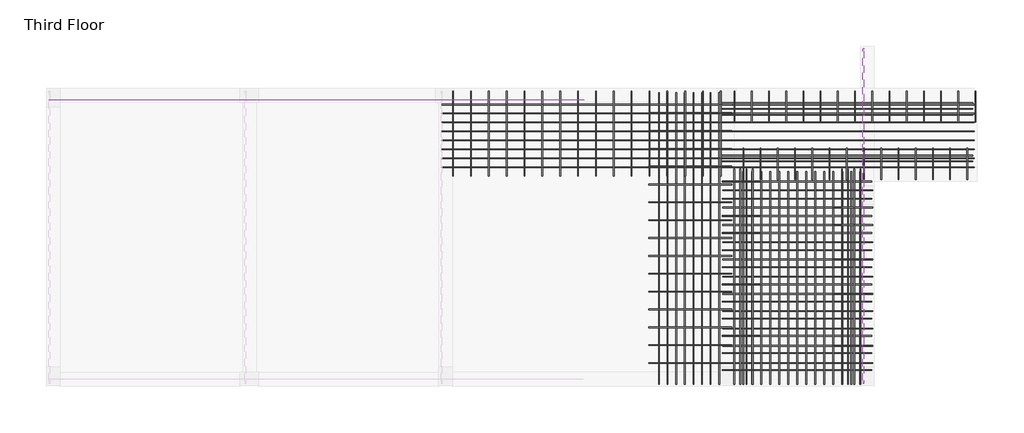
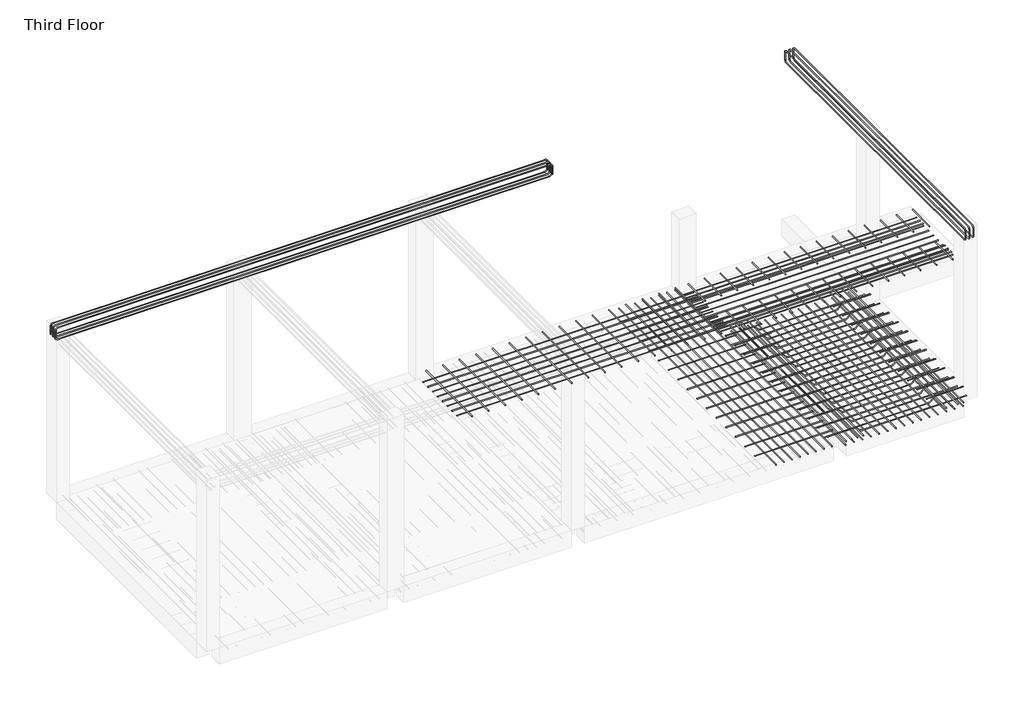
# One storey, part 4 of 4: 20 reinforcing bars.
"""IFC4 building model written with IfcOpenShell, lengths in millimetres."""

from ifc_helpers import new_model, si_unit, point, frame, origin, place, context, project, spatial, polyline, circle_curve, trimmed, segment, composite_curve, source, transform, mapped, element, save
from ifc_brep_helpers import swept_disk

model = new_model("IFC4")

# Units and contexts
model_context = context("Model", 3, world=origin())
ifc_project = project(units=[si_unit("LENGTHUNIT", "METRE", prefix="MILLI")], contexts=[model_context])

# Site, building, storey
site = spatial("IfcSite", under=ifc_project)
building = spatial("IfcBuilding", under=site)
storey = spatial("IfcBuildingStorey", under=building, Name="Third Floor", Elevation=9601.2)

# Reinforcing bars
placement = place(None, origin())
reinforcing_bar_shape = source(origin(), model_context, "Body", "SolidModel", [
    swept_disk(composite_curve([segment(polyline([(3999.1887526, 5724.7334631, 12564.4994949), (3999.1887526, 5724.7334631, 12712.4994949)]), True, "CONTINUOUS"), segment(trimmed(circle_curve(frame((3999.1887526, 5678.7334631, 12712.4994949), z_axis=(1.0, 0.0, 0.0), x_axis=(0.0, 46.0, 0.0)), 46.0), [point((3999.1887526, 5724.7334631, 12712.4994949))], [point((3999.1887526, 5678.7334631, 12758.4994949))], True, "CARTESIAN"), True, "CONTINUOUS"), segment(polyline([(3999.1887526, 5678.7334631, 12758.4994949), (3999.1887526, 278.4334631, 12758.4994949)]), True, "CONTINUOUS"), segment(trimmed(circle_curve(frame((3999.1887526, 278.4334631, 12712.4994949), z_axis=(1.0, 0.0, 0.0), x_axis=(0.0, 0.0, 46.0)), 46.0), [point((3999.1887526, 278.4334631, 12758.4994949))], [point((3999.1887526, 232.4334631, 12712.4994949))], True, "CARTESIAN"), True, "CONTINUOUS"), segment(polyline([(3999.1887526, 232.4334631, 12712.4994949), (3999.1887526, 232.4334631, 12564.4994949)]), True, "CONTINUOUS")], self_intersect=False), 6.0),
])
element("IfcReinforcingBar", 1, at=placement, inside=storey, context=model_context, shape_type="MappedRepresentation", body=[
    mapped(reinforcing_bar_shape, transform((0.0, 0.0, 0.0), x_axis=(1.0, 0.0, 0.0), y_axis=(0.0, 1.0, 0.0), z_axis=(0.0, 0.0, 1.0))),
    mapped(reinforcing_bar_shape, transform((71.1994949, 0.0, 0.0), x_axis=(1.0, 0.0, 0.0), y_axis=(0.0, 1.0, 0.0), z_axis=(0.0, 0.0, 1.0))),
    mapped(reinforcing_bar_shape, transform((142.3989899, 0.0, 0.0), x_axis=(1.0, 0.0, 0.0), y_axis=(0.0, 1.0, 0.0), z_axis=(0.0, 0.0, 1.0))),
])
reinforcing_bar_2_shape = source(origin(), model_context, "Body", "SolidModel", [
    swept_disk(composite_curve([segment(polyline([(3999.1887526, 5724.7334631, 12733.9005051), (3999.1887526, 5724.7334631, 12585.9005051)]), True, "CONTINUOUS"), segment(trimmed(circle_curve(frame((3999.1887526, 5678.7334631, 12585.9005051), z_axis=(-1.0, 0.0, 0.0), x_axis=(0.0, 46.0, 0.0)), 46.0), [point((3999.1887526, 5724.7334631, 12585.9005051))], [point((3999.1887526, 5678.7334631, 12539.9005051))], True, "CARTESIAN"), True, "CONTINUOUS"), segment(polyline([(3999.1887526, 5678.7334631, 12539.9005051), (3999.1887526, 278.4334631, 12539.9005051)]), True, "CONTINUOUS"), segment(trimmed(circle_curve(frame((3999.1887526, 278.4334631, 12585.9005051), z_axis=(-1.0, 0.0, 0.0), x_axis=(0.0, 0.0, -46.0)), 46.0), [point((3999.1887526, 278.4334631, 12539.9005051))], [point((3999.1887526, 232.4334631, 12585.9005051))], True, "CARTESIAN"), True, "CONTINUOUS"), segment(polyline([(3999.1887526, 232.4334631, 12585.9005051), (3999.1887526, 232.4334631, 12733.9005051)]), True, "CONTINUOUS")], self_intersect=False), 6.0),
])
element("IfcReinforcingBar", 2, at=placement, inside=storey, context=model_context, shape_type="MappedRepresentation", body=[
    mapped(reinforcing_bar_2_shape, transform((0.0, 0.0, 0.0), x_axis=(1.0, 0.0, 0.0), y_axis=(0.0, 1.0, 0.0), z_axis=(0.0, 0.0, 1.0))),
    mapped(reinforcing_bar_2_shape, transform((71.1994949, 0.0, 0.0), x_axis=(1.0, 0.0, 0.0), y_axis=(0.0, 1.0, 0.0), z_axis=(0.0, 0.0, 1.0))),
    mapped(reinforcing_bar_2_shape, transform((142.3989899, 0.0, 0.0), x_axis=(1.0, 0.0, 0.0), y_axis=(0.0, 1.0, 0.0), z_axis=(0.0, 0.0, 1.0))),
])
reinforcing_bar_3_shape = source(origin(), model_context, "Body", "SolidModel", [
    swept_disk(composite_curve([segment(polyline([(-586.8295875, 5020.132958, 12564.4994949), (-586.8295875, 5020.132958, 12712.4994949)]), True, "CONTINUOUS"), segment(trimmed(circle_curve(frame((-632.8295875, 5020.132958, 12712.4994949), z_axis=(0.0, -1.0, 0.0), x_axis=(46.0, 0.0, 0.0)), 46.0), [point((-586.8295875, 5020.132958, 12712.4994949))], [point((-632.8295875, 5020.132958, 12758.4994949))], True, "CARTESIAN"), True, "CONTINUOUS"), segment(polyline([(-632.8295875, 5020.132958, 12758.4994949), (-9286.9117524, 5020.132958, 12758.4994949)]), True, "CONTINUOUS"), segment(trimmed(circle_curve(frame((-9286.9117524, 5020.132958, 12712.4994949), z_axis=(0.0, -1.0, 0.0), x_axis=(0.0, 0.0, 46.0)), 46.0), [point((-9286.9117524, 5020.132958, 12758.4994949))], [point((-9332.9117524, 5020.132958, 12712.4994949))], True, "CARTESIAN"), True, "CONTINUOUS"), segment(polyline([(-9332.9117524, 5020.132958, 12712.4994949), (-9332.9117524, 5020.132958, 12564.4994949)]), True, "CONTINUOUS")], self_intersect=False), 6.0),
])
element("IfcReinforcingBar", 3, at=placement, inside=storey, context=model_context, shape_type="MappedRepresentation", body=[
    mapped(reinforcing_bar_3_shape, transform((0.0, 0.0, 0.0), x_axis=(1.0, 0.0, 0.0), y_axis=(0.0, 1.0, 0.0), z_axis=(0.0, 0.0, 1.0))),
    mapped(reinforcing_bar_3_shape, transform((0.0, -71.1994949, 0.0), x_axis=(1.0, 0.0, 0.0), y_axis=(0.0, 1.0, 0.0), z_axis=(0.0, 0.0, 1.0))),
    mapped(reinforcing_bar_3_shape, transform((0.0, -142.3989899, 0.0), x_axis=(1.0, 0.0, 0.0), y_axis=(0.0, 1.0, 0.0), z_axis=(0.0, 0.0, 1.0))),
])
reinforcing_bar_4_shape = source(origin(), model_context, "Body", "SolidModel", [
    swept_disk(composite_curve([segment(polyline([(-596.1117524, 5020.132958, 12733.9005051), (-596.1117524, 5020.132958, 12585.9005051)]), True, "CONTINUOUS"), segment(trimmed(circle_curve(frame((-642.1117524, 5020.132958, 12585.9005051), z_axis=(0.0, 1.0, 0.0), x_axis=(46.0, 0.0, 0.0)), 46.0), [point((-596.1117524, 5020.132958, 12585.9005051))], [point((-642.1117524, 5020.132958, 12539.9005051))], True, "CARTESIAN"), True, "CONTINUOUS"), segment(polyline([(-642.1117524, 5020.132958, 12539.9005051), (-9277.4938356, 5020.132958, 12539.9005051)]), True, "CONTINUOUS"), segment(trimmed(circle_curve(frame((-9277.4938356, 5020.132958, 12585.9005051), z_axis=(0.0, 1.0, 0.0), x_axis=(0.0, 0.0, -46.0)), 46.0), [point((-9277.4938356, 5020.132958, 12539.9005051))], [point((-9323.4938356, 5020.132958, 12585.9005051))], True, "CARTESIAN"), True, "CONTINUOUS"), segment(polyline([(-9323.4938356, 5020.132958, 12585.9005051), (-9323.4938356, 5020.132958, 12733.9005051)]), True, "CONTINUOUS")], self_intersect=False), 6.0),
])
element("IfcReinforcingBar", 4, at=placement, inside=storey, context=model_context, shape_type="MappedRepresentation", body=[
    mapped(reinforcing_bar_4_shape, transform((0.0, 0.0, 0.0), x_axis=(1.0, 0.0, 0.0), y_axis=(0.0, 1.0, 0.0), z_axis=(0.0, 0.0, 1.0))),
    mapped(reinforcing_bar_4_shape, transform((0.0, -71.1994949, 0.0), x_axis=(1.0, 0.0, 0.0), y_axis=(0.0, 1.0, 0.0), z_axis=(0.0, 0.0, 1.0))),
    mapped(reinforcing_bar_4_shape, transform((0.0, -142.3989899, 0.0), x_axis=(1.0, 0.0, 0.0), y_axis=(0.0, 1.0, 0.0), z_axis=(0.0, 0.0, 1.0))),
])
reinforcing_bar_5_shape = source(origin(), model_context, "Body", "SolidModel", [
    swept_disk(composite_curve([segment(polyline([(1688.7874305, 3539.2334631, 9570.2), (2168.5956769, 3539.2334631, 9570.2)]), True, "CONTINUOUS"), segment(trimmed(circle_curve(frame((2168.5956769, 3539.2334631, 9524.2), z_axis=(0.0, 1.0, 0.0), x_axis=(0.0, 0.0, 46.0)), 46.0), [point((2168.5956769, 3539.2334631, 9570.2))], [point((2201.1225888, 3539.2334631, 9556.7269119))], True, "CARTESIAN"), True, "CONTINUOUS"), segment(polyline([(2201.1225888, 3539.2334631, 9556.7269119), (2264.5764127, 3539.2334631, 9493.2730881)]), True, "CONTINUOUS"), segment(trimmed(circle_curve(frame((2297.1033246, 3539.2334631, 9525.8), z_axis=(0.0, -1.0, 0.0), x_axis=(-32.52691189999996, 0.0, -32.526911899998595)), 46.0), [point((2264.5764127, 3539.2334631, 9493.2730881))], [point((2297.1033246, 3539.2334631, 9479.8))], True, "CARTESIAN"), True, "CONTINUOUS"), segment(polyline([(2297.1033246, 3539.2334631, 9479.8), (4139.8402551, 3539.2334631, 9479.8)]), True, "CONTINUOUS")], self_intersect=False), 6.0),
])
element("IfcReinforcingBar", 5, at=placement, inside=storey, context=model_context, shape_type="MappedRepresentation", body=[
    mapped(reinforcing_bar_5_shape, transform((0.0, 0.0, 0.0), x_axis=(1.0, 0.0, 0.0), y_axis=(0.0, 1.0, 0.0), z_axis=(0.0, 0.0, 1.0))),
    mapped(reinforcing_bar_5_shape, transform((0.0, -281.0909091, 0.0), x_axis=(1.0, 0.0, 0.0), y_axis=(0.0, 1.0, 0.0), z_axis=(0.0, 0.0, 1.0))),
    mapped(reinforcing_bar_5_shape, transform((0.0, -562.1818182, 0.0), x_axis=(1.0, 0.0, 0.0), y_axis=(0.0, 1.0, 0.0), z_axis=(0.0, 0.0, 1.0))),
    mapped(reinforcing_bar_5_shape, transform((0.0, -843.2727273, 0.0), x_axis=(1.0, 0.0, 0.0), y_axis=(0.0, 1.0, 0.0), z_axis=(0.0, 0.0, 1.0))),
    mapped(reinforcing_bar_5_shape, transform((0.0, -1124.3636364, 0.0), x_axis=(1.0, 0.0, 0.0), y_axis=(0.0, 1.0, 0.0), z_axis=(0.0, 0.0, 1.0))),
    mapped(reinforcing_bar_5_shape, transform((0.0, -1405.4545455, 0.0), x_axis=(1.0, 0.0, 0.0), y_axis=(0.0, 1.0, 0.0), z_axis=(0.0, 0.0, 1.0))),
    mapped(reinforcing_bar_5_shape, transform((0.0, -1686.5454545, 0.0), x_axis=(1.0, 0.0, 0.0), y_axis=(0.0, 1.0, 0.0), z_axis=(0.0, 0.0, 1.0))),
    mapped(reinforcing_bar_5_shape, transform((0.0, -1967.6363636, 0.0), x_axis=(1.0, 0.0, 0.0), y_axis=(0.0, 1.0, 0.0), z_axis=(0.0, 0.0, 1.0))),
    mapped(reinforcing_bar_5_shape, transform((0.0, -2248.7272727, 0.0), x_axis=(1.0, 0.0, 0.0), y_axis=(0.0, 1.0, 0.0), z_axis=(0.0, 0.0, 1.0))),
    mapped(reinforcing_bar_5_shape, transform((0.0, -2529.8181818, 0.0), x_axis=(1.0, 0.0, 0.0), y_axis=(0.0, 1.0, 0.0), z_axis=(0.0, 0.0, 1.0))),
    mapped(reinforcing_bar_5_shape, transform((0.0, -2810.9090909, 0.0), x_axis=(1.0, 0.0, 0.0), y_axis=(0.0, 1.0, 0.0), z_axis=(0.0, 0.0, 1.0))),
    mapped(reinforcing_bar_5_shape, transform((0.0, -3092.0, 0.0), x_axis=(1.0, 0.0, 0.0), y_axis=(0.0, 1.0, 0.0), z_axis=(0.0, 0.0, 1.0))),
])
reinforcing_bar_6_shape = source(origin(), model_context, "Body", "SolidModel", [
    swept_disk(composite_curve([segment(polyline([(4153.2890646, 564.2307141, 9570.2), (3672.2951557, 564.2307141, 9570.2)]), True, "CONTINUOUS"), segment(trimmed(circle_curve(frame((3672.2951557, 564.2307141, 9524.2), z_axis=(0.0, -1.0, 0.0), x_axis=(0.0, 0.0, 46.0)), 46.0), [point((3672.2951557, 564.2307141, 9570.2))], [point((3639.7682438, 564.2307141, 9556.7269119))], True, "CARTESIAN"), True, "CONTINUOUS"), segment(polyline([(3639.7682438, 564.2307141, 9556.7269119), (3576.3144199, 564.2307141, 9493.2730881)]), True, "CONTINUOUS"), segment(trimmed(circle_curve(frame((3543.787508, 564.2307141, 9525.8), z_axis=(0.0, 1.0000000000000002, 0.0), x_axis=(32.52691189999996, 0.0, -32.526911899998595)), 46.0), [point((3576.3144199, 564.2307141, 9493.2730881))], [point((3543.787508, 564.2307141, 9479.8))], True, "CARTESIAN"), True, "CONTINUOUS"), segment(polyline([(3543.787508, 564.2307141, 9479.8), (1702.23624, 564.2307141, 9479.8)]), True, "CONTINUOUS")], self_intersect=False), 6.0),
])
element("IfcReinforcingBar", 6, at=placement, inside=storey, context=model_context, shape_type="MappedRepresentation", body=[
    mapped(reinforcing_bar_6_shape, transform((0.0, 0.0, 0.0), x_axis=(1.0, 0.0, 0.0), y_axis=(0.0, 1.0, 0.0), z_axis=(0.0, 0.0, 1.0))),
    mapped(reinforcing_bar_6_shape, transform((0.0, 283.1945647, 0.0), x_axis=(1.0, 0.0, 0.0), y_axis=(0.0, 1.0, 0.0), z_axis=(0.0, 0.0, 1.0))),
    mapped(reinforcing_bar_6_shape, transform((0.0, 566.3891295, 0.0), x_axis=(1.0, 0.0, 0.0), y_axis=(0.0, 1.0, 0.0), z_axis=(0.0, 0.0, 1.0))),
    mapped(reinforcing_bar_6_shape, transform((0.0, 849.5836942, 0.0), x_axis=(1.0, 0.0, 0.0), y_axis=(0.0, 1.0, 0.0), z_axis=(0.0, 0.0, 1.0))),
    mapped(reinforcing_bar_6_shape, transform((0.0, 1132.778259, 0.0), x_axis=(1.0, 0.0, 0.0), y_axis=(0.0, 1.0, 0.0), z_axis=(0.0, 0.0, 1.0))),
    mapped(reinforcing_bar_6_shape, transform((0.0, 1415.9728237, 0.0), x_axis=(1.0, 0.0, 0.0), y_axis=(0.0, 1.0, 0.0), z_axis=(0.0, 0.0, 1.0))),
    mapped(reinforcing_bar_6_shape, transform((0.0, 1699.1673885, 0.0), x_axis=(1.0, 0.0, 0.0), y_axis=(0.0, 1.0, 0.0), z_axis=(0.0, 0.0, 1.0))),
    mapped(reinforcing_bar_6_shape, transform((0.0, 1982.3619532, 0.0), x_axis=(1.0, 0.0, 0.0), y_axis=(0.0, 1.0, 0.0), z_axis=(0.0, 0.0, 1.0))),
    mapped(reinforcing_bar_6_shape, transform((0.0, 2265.556518, 0.0), x_axis=(1.0, 0.0, 0.0), y_axis=(0.0, 1.0, 0.0), z_axis=(0.0, 0.0, 1.0))),
    mapped(reinforcing_bar_6_shape, transform((0.0, 2548.7510827, 0.0), x_axis=(1.0, 0.0, 0.0), y_axis=(0.0, 1.0, 0.0), z_axis=(0.0, 0.0, 1.0))),
    mapped(reinforcing_bar_6_shape, transform((0.0, 2831.9456475, 0.0), x_axis=(1.0, 0.0, 0.0), y_axis=(0.0, 1.0, 0.0), z_axis=(0.0, 0.0, 1.0))),
])
reinforcing_bar_7_shape = source(origin(), model_context, "Body", "SolidModel", [
    swept_disk(composite_curve([segment(polyline([(3650.7560505, 3742.8334631, 9559.9006995), (3650.7560505, 211.4334631, 9559.9006995)]), True, "CONTINUOUS")], self_intersect=False), 6.0),
])
element("IfcReinforcingBar", 7, at=placement, inside=storey, context=model_context, shape_type="MappedRepresentation", body=[
    mapped(reinforcing_bar_7_shape, transform((0.0, 0.0, 0.0), x_axis=(1.0, 0.0, 0.0), y_axis=(0.0, 1.0, 0.0), z_axis=(0.0, 0.0, 1.0))),
    mapped(reinforcing_bar_7_shape, transform((101.777399, 0.0, 0.0), x_axis=(1.0, 0.0, 0.0), y_axis=(0.0, 1.0, 0.0), z_axis=(0.0, 0.0, 1.0))),
    mapped(reinforcing_bar_7_shape, transform((203.554798, 0.0, 0.0), x_axis=(1.0, 0.0, 0.0), y_axis=(0.0, 1.0, 0.0), z_axis=(0.0, 0.0, 1.0))),
    mapped(reinforcing_bar_7_shape, transform((305.3321971, 0.0, 0.0), x_axis=(1.0, 0.0, 0.0), y_axis=(0.0, 1.0, 0.0), z_axis=(0.0, 0.0, 1.0))),
])
reinforcing_bar_8_shape = source(origin(), model_context, "Body", "SolidModel", [
    swept_disk(composite_curve([segment(polyline([(1697.8477074, 3539.2334631, 9572.2), (2325.3671503, 3539.2334631, 9572.2)]), True, "CONTINUOUS")], self_intersect=False), 4.0),
])
element("IfcReinforcingBar", 8, at=placement, inside=storey, context=model_context, shape_type="MappedRepresentation", body=[
    mapped(reinforcing_bar_8_shape, transform((0.0, 0.0, 0.0), x_axis=(1.0, 0.0, 0.0), y_axis=(0.0, 1.0, 0.0), z_axis=(0.0, 0.0, 1.0))),
    mapped(reinforcing_bar_8_shape, transform((0.0, -281.0909091, 0.0), x_axis=(1.0, 0.0, 0.0), y_axis=(0.0, 1.0, 0.0), z_axis=(0.0, 0.0, 1.0))),
    mapped(reinforcing_bar_8_shape, transform((0.0, -562.1818182, 0.0), x_axis=(1.0, 0.0, 0.0), y_axis=(0.0, 1.0, 0.0), z_axis=(0.0, 0.0, 1.0))),
    mapped(reinforcing_bar_8_shape, transform((0.0, -843.2727273, 0.0), x_axis=(1.0, 0.0, 0.0), y_axis=(0.0, 1.0, 0.0), z_axis=(0.0, 0.0, 1.0))),
    mapped(reinforcing_bar_8_shape, transform((0.0, -1124.3636364, 0.0), x_axis=(1.0, 0.0, 0.0), y_axis=(0.0, 1.0, 0.0), z_axis=(0.0, 0.0, 1.0))),
    mapped(reinforcing_bar_8_shape, transform((0.0, -1405.4545455, 0.0), x_axis=(1.0, 0.0, 0.0), y_axis=(0.0, 1.0, 0.0), z_axis=(0.0, 0.0, 1.0))),
    mapped(reinforcing_bar_8_shape, transform((0.0, -1686.5454545, 0.0), x_axis=(1.0, 0.0, 0.0), y_axis=(0.0, 1.0, 0.0), z_axis=(0.0, 0.0, 1.0))),
    mapped(reinforcing_bar_8_shape, transform((0.0, -1967.6363636, 0.0), x_axis=(1.0, 0.0, 0.0), y_axis=(0.0, 1.0, 0.0), z_axis=(0.0, 0.0, 1.0))),
    mapped(reinforcing_bar_8_shape, transform((0.0, -2248.7272727, 0.0), x_axis=(1.0, 0.0, 0.0), y_axis=(0.0, 1.0, 0.0), z_axis=(0.0, 0.0, 1.0))),
    mapped(reinforcing_bar_8_shape, transform((0.0, -2529.8181818, 0.0), x_axis=(1.0, 0.0, 0.0), y_axis=(0.0, 1.0, 0.0), z_axis=(0.0, 0.0, 1.0))),
    mapped(reinforcing_bar_8_shape, transform((0.0, -2810.9090909, 0.0), x_axis=(1.0, 0.0, 0.0), y_axis=(0.0, 1.0, 0.0), z_axis=(0.0, 0.0, 1.0))),
    mapped(reinforcing_bar_8_shape, transform((0.0, -3092.0, 0.0), x_axis=(1.0, 0.0, 0.0), y_axis=(0.0, 1.0, 0.0), z_axis=(0.0, 0.0, 1.0))),
])
reinforcing_bar_9_shape = source(origin(), model_context, "Body", "SolidModel", [
    swept_disk(composite_curve([segment(polyline([(4130.5876361, 3396.1763616, 9572.2), (3500.3340616, 3396.1763616, 9572.2)]), True, "CONTINUOUS")], self_intersect=False), 4.0),
])
element("IfcReinforcingBar", 9, at=placement, inside=storey, context=model_context, shape_type="MappedRepresentation", body=[
    mapped(reinforcing_bar_9_shape, transform((0.0, 0.0, 0.0), x_axis=(1.0, 0.0, 0.0), y_axis=(0.0, 1.0, 0.0), z_axis=(0.0, 0.0, 1.0))),
    mapped(reinforcing_bar_9_shape, transform((0.0, -283.1945647, 0.0), x_axis=(1.0, 0.0, 0.0), y_axis=(0.0, 1.0, 0.0), z_axis=(0.0, 0.0, 1.0))),
    mapped(reinforcing_bar_9_shape, transform((0.0, -566.3891295, 0.0), x_axis=(1.0, 0.0, 0.0), y_axis=(0.0, 1.0, 0.0), z_axis=(0.0, 0.0, 1.0))),
    mapped(reinforcing_bar_9_shape, transform((0.0, -849.5836942, 0.0), x_axis=(1.0, 0.0, 0.0), y_axis=(0.0, 1.0, 0.0), z_axis=(0.0, 0.0, 1.0))),
    mapped(reinforcing_bar_9_shape, transform((0.0, -1132.778259, 0.0), x_axis=(1.0, 0.0, 0.0), y_axis=(0.0, 1.0, 0.0), z_axis=(0.0, 0.0, 1.0))),
    mapped(reinforcing_bar_9_shape, transform((0.0, -1415.9728237, 0.0), x_axis=(1.0, 0.0, 0.0), y_axis=(0.0, 1.0, 0.0), z_axis=(0.0, 0.0, 1.0))),
    mapped(reinforcing_bar_9_shape, transform((0.0, -1699.1673885, 0.0), x_axis=(1.0, 0.0, 0.0), y_axis=(0.0, 1.0, 0.0), z_axis=(0.0, 0.0, 1.0))),
    mapped(reinforcing_bar_9_shape, transform((0.0, -1982.3619532, 0.0), x_axis=(1.0, 0.0, 0.0), y_axis=(0.0, 1.0, 0.0), z_axis=(0.0, 0.0, 1.0))),
    mapped(reinforcing_bar_9_shape, transform((0.0, -2265.556518, 0.0), x_axis=(1.0, 0.0, 0.0), y_axis=(0.0, 1.0, 0.0), z_axis=(0.0, 0.0, 1.0))),
    mapped(reinforcing_bar_9_shape, transform((0.0, -2548.7510827, 0.0), x_axis=(1.0, 0.0, 0.0), y_axis=(0.0, 1.0, 0.0), z_axis=(0.0, 0.0, 1.0))),
    mapped(reinforcing_bar_9_shape, transform((0.0, -2831.9456475, 0.0), x_axis=(1.0, 0.0, 0.0), y_axis=(0.0, 1.0, 0.0), z_axis=(0.0, 0.0, 1.0))),
])
reinforcing_bar_10_shape = source(origin(), model_context, "Body", "SolidModel", [
    swept_disk(composite_curve([segment(polyline([(3952.0882476, 218.9117605, 9488.3387401), (3952.0882476, 3706.6679133, 9488.3387401)]), True, "CONTINUOUS")], self_intersect=False), 6.0),
])
element("IfcReinforcingBar", 10, at=placement, inside=storey, context=model_context, shape_type="MappedRepresentation", body=[
    mapped(reinforcing_bar_10_shape, transform((0.0, 0.0, 0.0), x_axis=(1.0, 0.0, 0.0), y_axis=(0.0, 1.0, 0.0), z_axis=(0.0, 0.0, 1.0))),
    mapped(reinforcing_bar_10_shape, transform((-147.5785714, 0.0, 0.0), x_axis=(1.0, 0.0, 0.0), y_axis=(0.0, 1.0, 0.0), z_axis=(0.0, 0.0, 1.0))),
    mapped(reinforcing_bar_10_shape, transform((-295.1571429, 0.0, 0.0), x_axis=(1.0, 0.0, 0.0), y_axis=(0.0, 1.0, 0.0), z_axis=(0.0, 0.0, 1.0))),
    mapped(reinforcing_bar_10_shape, transform((-442.7357143, 0.0, 0.0), x_axis=(1.0, 0.0, 0.0), y_axis=(0.0, 1.0, 0.0), z_axis=(0.0, 0.0, 1.0))),
    mapped(reinforcing_bar_10_shape, transform((-590.3142857, 0.0, 0.0), x_axis=(1.0, 0.0, 0.0), y_axis=(0.0, 1.0, 0.0), z_axis=(0.0, 0.0, 1.0))),
    mapped(reinforcing_bar_10_shape, transform((-737.8928571, 0.0, 0.0), x_axis=(1.0, 0.0, 0.0), y_axis=(0.0, 1.0, 0.0), z_axis=(0.0, 0.0, 1.0))),
    mapped(reinforcing_bar_10_shape, transform((-885.4714286, 0.0, 0.0), x_axis=(1.0, 0.0, 0.0), y_axis=(0.0, 1.0, 0.0), z_axis=(0.0, 0.0, 1.0))),
    mapped(reinforcing_bar_10_shape, transform((-1033.05, 0.0, 0.0), x_axis=(1.0, 0.0, 0.0), y_axis=(0.0, 1.0, 0.0), z_axis=(0.0, 0.0, 1.0))),
    mapped(reinforcing_bar_10_shape, transform((-1180.6285714, 0.0, 0.0), x_axis=(1.0, 0.0, 0.0), y_axis=(0.0, 1.0, 0.0), z_axis=(0.0, 0.0, 1.0))),
    mapped(reinforcing_bar_10_shape, transform((-1328.2071429, 0.0, 0.0), x_axis=(1.0, 0.0, 0.0), y_axis=(0.0, 1.0, 0.0), z_axis=(0.0, 0.0, 1.0))),
    mapped(reinforcing_bar_10_shape, transform((-1475.7857143, 0.0, 0.0), x_axis=(1.0, 0.0, 0.0), y_axis=(0.0, 1.0, 0.0), z_axis=(0.0, 0.0, 1.0))),
    mapped(reinforcing_bar_10_shape, transform((-1623.3642857, 0.0, 0.0), x_axis=(1.0, 0.0, 0.0), y_axis=(0.0, 1.0, 0.0), z_axis=(0.0, 0.0, 1.0))),
    mapped(reinforcing_bar_10_shape, transform((-1770.9428571, 0.0, 0.0), x_axis=(1.0, 0.0, 0.0), y_axis=(0.0, 1.0, 0.0), z_axis=(0.0, 0.0, 1.0))),
    mapped(reinforcing_bar_10_shape, transform((-1918.5214286, 0.0, 0.0), x_axis=(1.0, 0.0, 0.0), y_axis=(0.0, 1.0, 0.0), z_axis=(0.0, 0.0, 1.0))),
    mapped(reinforcing_bar_10_shape, transform((-2066.1, 0.0, 0.0), x_axis=(1.0, 0.0, 0.0), y_axis=(0.0, 1.0, 0.0), z_axis=(0.0, 0.0, 1.0))),
])
reinforcing_bar_11_shape = source(origin(), model_context, "Body", "SolidModel", [
    swept_disk(composite_curve([segment(polyline([(2190.1347821, 3742.8334631, 9559.9006995), (2190.1347821, 211.4334631, 9559.9006995)]), True, "CONTINUOUS")], self_intersect=False), 6.0),
])
element("IfcReinforcingBar", 11, at=placement, inside=storey, context=model_context, shape_type="MappedRepresentation", body=[
    mapped(reinforcing_bar_11_shape, transform((0.0, 0.0, 0.0), x_axis=(1.0, 0.0, 0.0), y_axis=(0.0, 1.0, 0.0), z_axis=(0.0, 0.0, 1.0))),
    mapped(reinforcing_bar_11_shape, transform((-101.3821782, 0.0, 0.0), x_axis=(1.0, 0.0, 0.0), y_axis=(0.0, 1.0, 0.0), z_axis=(0.0, 0.0, 1.0))),
    mapped(reinforcing_bar_11_shape, transform((-202.7643564, 0.0, 0.0), x_axis=(1.0, 0.0, 0.0), y_axis=(0.0, 1.0, 0.0), z_axis=(0.0, 0.0, 1.0))),
    mapped(reinforcing_bar_11_shape, transform((-304.1465345, 0.0, 0.0), x_axis=(1.0, 0.0, 0.0), y_axis=(0.0, 1.0, 0.0), z_axis=(0.0, 0.0, 1.0))),
])
reinforcing_bar_12_shape = source(origin(), model_context, "Body", "SolidModel", [
    swept_disk(composite_curve([segment(polyline([(654.4332967, 4999.0798317, 9555.2697281), (654.4332967, 211.4334631, 9555.2697281)]), True, "CONTINUOUS")], self_intersect=False), 6.0),
])
element("IfcReinforcingBar", 12, at=placement, inside=storey, context=model_context, shape_type="MappedRepresentation", body=[
    mapped(reinforcing_bar_12_shape, transform((0.0, 0.0, 0.0), x_axis=(1.0, 0.0, 0.0), y_axis=(0.0, 1.0, 0.0), z_axis=(0.0, 0.0, 1.0))),
    mapped(reinforcing_bar_12_shape, transform((140.8412233, 0.0, 0.0), x_axis=(1.0, 0.0, 0.0), y_axis=(0.0, 1.0, 0.0), z_axis=(0.0, 0.0, 1.0))),
    mapped(reinforcing_bar_12_shape, transform((281.6824466, 0.0, 0.0), x_axis=(1.0, 0.0, 0.0), y_axis=(0.0, 1.0, 0.0), z_axis=(0.0, 0.0, 1.0))),
    mapped(reinforcing_bar_12_shape, transform((422.5236699, 0.0, 0.0), x_axis=(1.0, 0.0, 0.0), y_axis=(0.0, 1.0, 0.0), z_axis=(0.0, 0.0, 1.0))),
    mapped(reinforcing_bar_12_shape, transform((563.3648932, 0.0, 0.0), x_axis=(1.0, 0.0, 0.0), y_axis=(0.0, 1.0, 0.0), z_axis=(0.0, 0.0, 1.0))),
    mapped(reinforcing_bar_12_shape, transform((704.2061164, 0.0, 0.0), x_axis=(1.0, 0.0, 0.0), y_axis=(0.0, 1.0, 0.0), z_axis=(0.0, 0.0, 1.0))),
    mapped(reinforcing_bar_12_shape, transform((845.0473397, 0.0, 0.0), x_axis=(1.0, 0.0, 0.0), y_axis=(0.0, 1.0, 0.0), z_axis=(0.0, 0.0, 1.0))),
    mapped(reinforcing_bar_12_shape, transform((985.888563, 0.0, 0.0), x_axis=(1.0, 0.0, 0.0), y_axis=(0.0, 1.0, 0.0), z_axis=(0.0, 0.0, 1.0))),
])
reinforcing_bar_13_shape = source(origin(), model_context, "Body", "SolidModel", [
    swept_disk(composite_curve([segment(polyline([(1844.9074635, 564.2307141, 9564.6017937), (483.2910842, 564.2307141, 9564.6017937)]), True, "CONTINUOUS")], self_intersect=False), 6.0),
])
element("IfcReinforcingBar", 13, at=placement, inside=storey, context=model_context, shape_type="MappedRepresentation", body=[
    mapped(reinforcing_bar_13_shape, transform((0.0, 0.0, 0.0), x_axis=(1.0, 0.0, 0.0), y_axis=(0.0, 1.0, 0.0), z_axis=(0.0, 0.0, 1.0))),
    mapped(reinforcing_bar_13_shape, transform((0.0, 292.7783831, 0.0), x_axis=(1.0, 0.0, 0.0), y_axis=(0.0, 1.0, 0.0), z_axis=(0.0, 0.0, 1.0))),
    mapped(reinforcing_bar_13_shape, transform((0.0, 585.5567661, 0.0), x_axis=(1.0, 0.0, 0.0), y_axis=(0.0, 1.0, 0.0), z_axis=(0.0, 0.0, 1.0))),
    mapped(reinforcing_bar_13_shape, transform((0.0, 878.3351492, 0.0), x_axis=(1.0, 0.0, 0.0), y_axis=(0.0, 1.0, 0.0), z_axis=(0.0, 0.0, 1.0))),
    mapped(reinforcing_bar_13_shape, transform((0.0, 1171.1135323, 0.0), x_axis=(1.0, 0.0, 0.0), y_axis=(0.0, 1.0, 0.0), z_axis=(0.0, 0.0, 1.0))),
    mapped(reinforcing_bar_13_shape, transform((0.0, 1463.8919154, 0.0), x_axis=(1.0, 0.0, 0.0), y_axis=(0.0, 1.0, 0.0), z_axis=(0.0, 0.0, 1.0))),
    mapped(reinforcing_bar_13_shape, transform((0.0, 1756.6702984, 0.0), x_axis=(1.0, 0.0, 0.0), y_axis=(0.0, 1.0, 0.0), z_axis=(0.0, 0.0, 1.0))),
    mapped(reinforcing_bar_13_shape, transform((0.0, 2049.4486815, 0.0), x_axis=(1.0, 0.0, 0.0), y_axis=(0.0, 1.0, 0.0), z_axis=(0.0, 0.0, 1.0))),
    mapped(reinforcing_bar_13_shape, transform((0.0, 2342.2270646, 0.0), x_axis=(1.0, 0.0, 0.0), y_axis=(0.0, 1.0, 0.0), z_axis=(0.0, 0.0, 1.0))),
    mapped(reinforcing_bar_13_shape, transform((0.0, 2635.0054477, 0.0), x_axis=(1.0, 0.0, 0.0), y_axis=(0.0, 1.0, 0.0), z_axis=(0.0, 0.0, 1.0))),
    mapped(reinforcing_bar_13_shape, transform((0.0, 2927.7838307, 0.0), x_axis=(1.0, 0.0, 0.0), y_axis=(0.0, 1.0, 0.0), z_axis=(0.0, 0.0, 1.0))),
    mapped(reinforcing_bar_13_shape, transform((0.0, 3220.5622138, 0.0), x_axis=(1.0, 0.0, 0.0), y_axis=(0.0, 1.0, 0.0), z_axis=(0.0, 0.0, 1.0))),
    mapped(reinforcing_bar_13_shape, transform((0.0, 3513.3405969, 0.0), x_axis=(1.0, 0.0, 0.0), y_axis=(0.0, 1.0, 0.0), z_axis=(0.0, 0.0, 1.0))),
    mapped(reinforcing_bar_13_shape, transform((0.0, 3806.11898, 0.0), x_axis=(1.0, 0.0, 0.0), y_axis=(0.0, 1.0, 0.0), z_axis=(0.0, 0.0, 1.0))),
    mapped(reinforcing_bar_13_shape, transform((0.0, 4098.897363, 0.0), x_axis=(1.0, 0.0, 0.0), y_axis=(0.0, 1.0, 0.0), z_axis=(0.0, 0.0, 1.0))),
])
reinforcing_bar_14_shape = source(origin(), model_context, "Body", "SolidModel", [
    swept_disk(composite_curve([segment(polyline([(1854.5084921, 3775.4003908, 9554.9006995), (-2903.4807845, 3775.4003908, 9554.9006995)]), True, "CONTINUOUS")], self_intersect=False), 6.0),
])
element("IfcReinforcingBar", 14, at=placement, inside=storey, context=model_context, shape_type="MappedRepresentation", body=[
    mapped(reinforcing_bar_14_shape, transform((0.0, 0.0, 0.0), x_axis=(1.0, 0.0, 0.0), y_axis=(0.0, 1.0, 0.0), z_axis=(0.0, 0.0, 1.0))),
    mapped(reinforcing_bar_14_shape, transform((0.0, 146.8904389, 0.0), x_axis=(1.0, 0.0, 0.0), y_axis=(0.0, 1.0, 0.0), z_axis=(0.0, 0.0, 1.0))),
    mapped(reinforcing_bar_14_shape, transform((0.0, 293.7808778, 0.0), x_axis=(1.0, 0.0, 0.0), y_axis=(0.0, 1.0, 0.0), z_axis=(0.0, 0.0, 1.0))),
    mapped(reinforcing_bar_14_shape, transform((0.0, 440.6713167, 0.0), x_axis=(1.0, 0.0, 0.0), y_axis=(0.0, 1.0, 0.0), z_axis=(0.0, 0.0, 1.0))),
    mapped(reinforcing_bar_14_shape, transform((0.0, 587.5617556, 0.0), x_axis=(1.0, 0.0, 0.0), y_axis=(0.0, 1.0, 0.0), z_axis=(0.0, 0.0, 1.0))),
    mapped(reinforcing_bar_14_shape, transform((0.0, 734.4521945, 0.0), x_axis=(1.0, 0.0, 0.0), y_axis=(0.0, 1.0, 0.0), z_axis=(0.0, 0.0, 1.0))),
    mapped(reinforcing_bar_14_shape, transform((0.0, 881.3426334, 0.0), x_axis=(1.0, 0.0, 0.0), y_axis=(0.0, 1.0, 0.0), z_axis=(0.0, 0.0, 1.0))),
    mapped(reinforcing_bar_14_shape, transform((0.0, 1028.2330723, 0.0), x_axis=(1.0, 0.0, 0.0), y_axis=(0.0, 1.0, 0.0), z_axis=(0.0, 0.0, 1.0))),
])
reinforcing_bar_15_shape = source(origin(), model_context, "Body", "SolidModel", [
    swept_disk(composite_curve([segment(polyline([(1667.8254733, 5026.3578219, 9564.6017937), (1667.8254733, 3630.6252123, 9564.6017937)]), True, "CONTINUOUS")], self_intersect=False), 6.0),
])
element("IfcReinforcingBar", 15, at=placement, inside=storey, context=model_context, shape_type="MappedRepresentation", body=[
    mapped(reinforcing_bar_15_shape, transform((0.0, 0.0, 0.0), x_axis=(1.0, 0.0, 0.0), y_axis=(0.0, 1.0, 0.0), z_axis=(0.0, 0.0, 1.0))),
    mapped(reinforcing_bar_15_shape, transform((-292.44, 0.0, 0.0), x_axis=(1.0, 0.0, 0.0), y_axis=(0.0, 1.0, 0.0), z_axis=(0.0, 0.0, 1.0))),
    mapped(reinforcing_bar_15_shape, transform((-584.88, 0.0, 0.0), x_axis=(1.0, 0.0, 0.0), y_axis=(0.0, 1.0, 0.0), z_axis=(0.0, 0.0, 1.0))),
    mapped(reinforcing_bar_15_shape, transform((-877.32, 0.0, 0.0), x_axis=(1.0, 0.0, 0.0), y_axis=(0.0, 1.0, 0.0), z_axis=(0.0, 0.0, 1.0))),
    mapped(reinforcing_bar_15_shape, transform((-1169.76, 0.0, 0.0), x_axis=(1.0, 0.0, 0.0), y_axis=(0.0, 1.0, 0.0), z_axis=(0.0, 0.0, 1.0))),
    mapped(reinforcing_bar_15_shape, transform((-1462.2, 0.0, 0.0), x_axis=(1.0, 0.0, 0.0), y_axis=(0.0, 1.0, 0.0), z_axis=(0.0, 0.0, 1.0))),
    mapped(reinforcing_bar_15_shape, transform((-1754.64, 0.0, 0.0), x_axis=(1.0, 0.0, 0.0), y_axis=(0.0, 1.0, 0.0), z_axis=(0.0, 0.0, 1.0))),
    mapped(reinforcing_bar_15_shape, transform((-2047.08, 0.0, 0.0), x_axis=(1.0, 0.0, 0.0), y_axis=(0.0, 1.0, 0.0), z_axis=(0.0, 0.0, 1.0))),
    mapped(reinforcing_bar_15_shape, transform((-2339.52, 0.0, 0.0), x_axis=(1.0, 0.0, 0.0), y_axis=(0.0, 1.0, 0.0), z_axis=(0.0, 0.0, 1.0))),
    mapped(reinforcing_bar_15_shape, transform((-2631.96, 0.0, 0.0), x_axis=(1.0, 0.0, 0.0), y_axis=(0.0, 1.0, 0.0), z_axis=(0.0, 0.0, 1.0))),
    mapped(reinforcing_bar_15_shape, transform((-2924.4, 0.0, 0.0), x_axis=(1.0, 0.0, 0.0), y_axis=(0.0, 1.0, 0.0), z_axis=(0.0, 0.0, 1.0))),
    mapped(reinforcing_bar_15_shape, transform((-3216.84, 0.0, 0.0), x_axis=(1.0, 0.0, 0.0), y_axis=(0.0, 1.0, 0.0), z_axis=(0.0, 0.0, 1.0))),
    mapped(reinforcing_bar_15_shape, transform((-3509.28, 0.0, 0.0), x_axis=(1.0, 0.0, 0.0), y_axis=(0.0, 1.0, 0.0), z_axis=(0.0, 0.0, 1.0))),
    mapped(reinforcing_bar_15_shape, transform((-3801.72, 0.0, 0.0), x_axis=(1.0, 0.0, 0.0), y_axis=(0.0, 1.0, 0.0), z_axis=(0.0, 0.0, 1.0))),
    mapped(reinforcing_bar_15_shape, transform((-4094.16, 0.0, 0.0), x_axis=(1.0, 0.0, 0.0), y_axis=(0.0, 1.0, 0.0), z_axis=(0.0, 0.0, 1.0))),
    mapped(reinforcing_bar_15_shape, transform((-4386.6, 0.0, 0.0), x_axis=(1.0, 0.0, 0.0), y_axis=(0.0, 1.0, 0.0), z_axis=(0.0, 0.0, 1.0))),
])
reinforcing_bar_16_shape = source(origin(), model_context, "Body", "SolidModel", [
    swept_disk(composite_curve([segment(polyline([(5796.3354159, 4634.2611065, 9555.1212824), (1682.3882476, 4634.2611065, 9555.1212824)]), True, "CONTINUOUS")], self_intersect=False), 6.0),
])
element("IfcReinforcingBar", 16, at=placement, inside=storey, context=model_context, shape_type="MappedRepresentation", body=[
    mapped(reinforcing_bar_16_shape, transform((0.0, 0.0, 0.0), x_axis=(1.0, 0.0, 0.0), y_axis=(0.0, 1.0, 0.0), z_axis=(0.0, 0.0, 1.0))),
    mapped(reinforcing_bar_16_shape, transform((0.0, 96.3869435, 0.0), x_axis=(1.0, 0.0, 0.0), y_axis=(0.0, 1.0, 0.0), z_axis=(0.0, 0.0, 1.0))),
    mapped(reinforcing_bar_16_shape, transform((0.0, 192.773887, 0.0), x_axis=(1.0, 0.0, 0.0), y_axis=(0.0, 1.0, 0.0), z_axis=(0.0, 0.0, 1.0))),
])
reinforcing_bar_17_shape = source(origin(), model_context, "Body", "SolidModel", [
    swept_disk(composite_curve([segment(polyline([(5798.6824692, 3968.2058196, 9555.1212824), (1682.3882476, 3968.2058196, 9555.1212824)]), True, "CONTINUOUS")], self_intersect=False), 6.0),
])
element("IfcReinforcingBar", 17, at=placement, inside=storey, context=model_context, shape_type="MappedRepresentation", body=[
    mapped(reinforcing_bar_17_shape, transform((0.0, 0.0, 0.0), x_axis=(1.0, 0.0, 0.0), y_axis=(0.0, 1.0, 0.0), z_axis=(0.0, 0.0, 1.0))),
    mapped(reinforcing_bar_17_shape, transform((0.0, -96.3869435, 0.0), x_axis=(1.0, 0.0, 0.0), y_axis=(0.0, 1.0, 0.0), z_axis=(0.0, 0.0, 1.0))),
    mapped(reinforcing_bar_17_shape, transform((0.0, -192.773887, 0.0), x_axis=(1.0, 0.0, 0.0), y_axis=(0.0, 1.0, 0.0), z_axis=(0.0, 0.0, 1.0))),
])
reinforcing_bar_18_shape = source(origin(), model_context, "Body", "SolidModel", [
    swept_disk(composite_curve([segment(polyline([(5840.6882476, 5026.8576948, 9563.3336733), (5840.6882476, 4511.8136411, 9563.3336733)]), True, "CONTINUOUS")], self_intersect=False), 6.0),
])
element("IfcReinforcingBar", 18, at=placement, inside=storey, context=model_context, shape_type="MappedRepresentation", body=[
    mapped(reinforcing_bar_18_shape, transform((0.0, 0.0, 0.0), x_axis=(1.0, 0.0, 0.0), y_axis=(0.0, 1.0, 0.0), z_axis=(0.0, 0.0, 1.0))),
    mapped(reinforcing_bar_18_shape, transform((-282.05, 0.0, 0.0), x_axis=(1.0, 0.0, 0.0), y_axis=(0.0, 1.0, 0.0), z_axis=(0.0, 0.0, 1.0))),
    mapped(reinforcing_bar_18_shape, transform((-564.1, 0.0, 0.0), x_axis=(1.0, 0.0, 0.0), y_axis=(0.0, 1.0, 0.0), z_axis=(0.0, 0.0, 1.0))),
    mapped(reinforcing_bar_18_shape, transform((-846.15, 0.0, 0.0), x_axis=(1.0, 0.0, 0.0), y_axis=(0.0, 1.0, 0.0), z_axis=(0.0, 0.0, 1.0))),
    mapped(reinforcing_bar_18_shape, transform((-1128.2, 0.0, 0.0), x_axis=(1.0, 0.0, 0.0), y_axis=(0.0, 1.0, 0.0), z_axis=(0.0, 0.0, 1.0))),
    mapped(reinforcing_bar_18_shape, transform((-1410.25, 0.0, 0.0), x_axis=(1.0, 0.0, 0.0), y_axis=(0.0, 1.0, 0.0), z_axis=(0.0, 0.0, 1.0))),
    mapped(reinforcing_bar_18_shape, transform((-1692.3, 0.0, 0.0), x_axis=(1.0, 0.0, 0.0), y_axis=(0.0, 1.0, 0.0), z_axis=(0.0, 0.0, 1.0))),
    mapped(reinforcing_bar_18_shape, transform((-1974.35, 0.0, 0.0), x_axis=(1.0, 0.0, 0.0), y_axis=(0.0, 1.0, 0.0), z_axis=(0.0, 0.0, 1.0))),
    mapped(reinforcing_bar_18_shape, transform((-2256.4, 0.0, 0.0), x_axis=(1.0, 0.0, 0.0), y_axis=(0.0, 1.0, 0.0), z_axis=(0.0, 0.0, 1.0))),
    mapped(reinforcing_bar_18_shape, transform((-2538.45, 0.0, 0.0), x_axis=(1.0, 0.0, 0.0), y_axis=(0.0, 1.0, 0.0), z_axis=(0.0, 0.0, 1.0))),
    mapped(reinforcing_bar_18_shape, transform((-2820.5, 0.0, 0.0), x_axis=(1.0, 0.0, 0.0), y_axis=(0.0, 1.0, 0.0), z_axis=(0.0, 0.0, 1.0))),
    mapped(reinforcing_bar_18_shape, transform((-3102.55, 0.0, 0.0), x_axis=(1.0, 0.0, 0.0), y_axis=(0.0, 1.0, 0.0), z_axis=(0.0, 0.0, 1.0))),
    mapped(reinforcing_bar_18_shape, transform((-3384.6, 0.0, 0.0), x_axis=(1.0, 0.0, 0.0), y_axis=(0.0, 1.0, 0.0), z_axis=(0.0, 0.0, 1.0))),
    mapped(reinforcing_bar_18_shape, transform((-3666.65, 0.0, 0.0), x_axis=(1.0, 0.0, 0.0), y_axis=(0.0, 1.0, 0.0), z_axis=(0.0, 0.0, 1.0))),
    mapped(reinforcing_bar_18_shape, transform((-3948.7, 0.0, 0.0), x_axis=(1.0, 0.0, 0.0), y_axis=(0.0, 1.0, 0.0), z_axis=(0.0, 0.0, 1.0))),
])
reinforcing_bar_19_shape = source(origin(), model_context, "Body", "SolidModel", [
    swept_disk(composite_curve([segment(polyline([(5706.0756595, 3575.6092313, 9563.3336733), (5706.0756595, 4090.653285, 9563.3336733)]), True, "CONTINUOUS")], self_intersect=False), 6.0),
])
element("IfcReinforcingBar", 19, at=placement, inside=storey, context=model_context, shape_type="MappedRepresentation", body=[
    mapped(reinforcing_bar_19_shape, transform((0.0, 0.0, 0.0), x_axis=(1.0, 0.0, 0.0), y_axis=(0.0, 1.0, 0.0), z_axis=(0.0, 0.0, 1.0))),
    mapped(reinforcing_bar_19_shape, transform((-282.2377571, 0.0, 0.0), x_axis=(1.0, 0.0, 0.0), y_axis=(0.0, 1.0, 0.0), z_axis=(0.0, 0.0, 1.0))),
    mapped(reinforcing_bar_19_shape, transform((-564.4755142, 0.0, 0.0), x_axis=(1.0, 0.0, 0.0), y_axis=(0.0, 1.0, 0.0), z_axis=(0.0, 0.0, 1.0))),
    mapped(reinforcing_bar_19_shape, transform((-846.7132714, 0.0, 0.0), x_axis=(1.0, 0.0, 0.0), y_axis=(0.0, 1.0, 0.0), z_axis=(0.0, 0.0, 1.0))),
    mapped(reinforcing_bar_19_shape, transform((-1128.9510285, 0.0, 0.0), x_axis=(1.0, 0.0, 0.0), y_axis=(0.0, 1.0, 0.0), z_axis=(0.0, 0.0, 1.0))),
    mapped(reinforcing_bar_19_shape, transform((-1411.1887856, 0.0, 0.0), x_axis=(1.0, 0.0, 0.0), y_axis=(0.0, 1.0, 0.0), z_axis=(0.0, 0.0, 1.0))),
    mapped(reinforcing_bar_19_shape, transform((-1693.4265427, 0.0, 0.0), x_axis=(1.0, 0.0, 0.0), y_axis=(0.0, 1.0, 0.0), z_axis=(0.0, 0.0, 1.0))),
    mapped(reinforcing_bar_19_shape, transform((-1975.6642999, 0.0, 0.0), x_axis=(1.0, 0.0, 0.0), y_axis=(0.0, 1.0, 0.0), z_axis=(0.0, 0.0, 1.0))),
    mapped(reinforcing_bar_19_shape, transform((-2257.902057, 0.0, 0.0), x_axis=(1.0, 0.0, 0.0), y_axis=(0.0, 1.0, 0.0), z_axis=(0.0, 0.0, 1.0))),
    mapped(reinforcing_bar_19_shape, transform((-2540.1398141, 0.0, 0.0), x_axis=(1.0, 0.0, 0.0), y_axis=(0.0, 1.0, 0.0), z_axis=(0.0, 0.0, 1.0))),
    mapped(reinforcing_bar_19_shape, transform((-2822.3775712, 0.0, 0.0), x_axis=(1.0, 0.0, 0.0), y_axis=(0.0, 1.0, 0.0), z_axis=(0.0, 0.0, 1.0))),
    mapped(reinforcing_bar_19_shape, transform((-3104.6153284, 0.0, 0.0), x_axis=(1.0, 0.0, 0.0), y_axis=(0.0, 1.0, 0.0), z_axis=(0.0, 0.0, 1.0))),
    mapped(reinforcing_bar_19_shape, transform((-3386.8530855, 0.0, 0.0), x_axis=(1.0, 0.0, 0.0), y_axis=(0.0, 1.0, 0.0), z_axis=(0.0, 0.0, 1.0))),
    mapped(reinforcing_bar_19_shape, transform((-3669.0908426, 0.0, 0.0), x_axis=(1.0, 0.0, 0.0), y_axis=(0.0, 1.0, 0.0), z_axis=(0.0, 0.0, 1.0))),
])
reinforcing_bar_20_shape = source(origin(), model_context, "Body", "SolidModel", [
    swept_disk(composite_curve([segment(polyline([(5819.6977393, 4803.6334631, 9493.6289517), (1682.3882476, 4803.6334631, 9493.6289517)]), True, "CONTINUOUS")], self_intersect=False), 6.0),
])
element("IfcReinforcingBar", 20, at=placement, inside=storey, context=model_context, shape_type="MappedRepresentation", body=[
    mapped(reinforcing_bar_20_shape, transform((0.0, 0.0, 0.0), x_axis=(1.0, 0.0, 0.0), y_axis=(0.0, 1.0, 0.0), z_axis=(0.0, 0.0, 1.0))),
    mapped(reinforcing_bar_20_shape, transform((0.0, -147.1142857, 0.0), x_axis=(1.0, 0.0, 0.0), y_axis=(0.0, 1.0, 0.0), z_axis=(0.0, 0.0, 1.0))),
    mapped(reinforcing_bar_20_shape, transform((0.0, -294.2285714, 0.0), x_axis=(1.0, 0.0, 0.0), y_axis=(0.0, 1.0, 0.0), z_axis=(0.0, 0.0, 1.0))),
    mapped(reinforcing_bar_20_shape, transform((0.0, -441.3428571, 0.0), x_axis=(1.0, 0.0, 0.0), y_axis=(0.0, 1.0, 0.0), z_axis=(0.0, 0.0, 1.0))),
    mapped(reinforcing_bar_20_shape, transform((0.0, -588.4571429, 0.0), x_axis=(1.0, 0.0, 0.0), y_axis=(0.0, 1.0, 0.0), z_axis=(0.0, 0.0, 1.0))),
    mapped(reinforcing_bar_20_shape, transform((0.0, -735.5714286, 0.0), x_axis=(1.0, 0.0, 0.0), y_axis=(0.0, 1.0, 0.0), z_axis=(0.0, 0.0, 1.0))),
    mapped(reinforcing_bar_20_shape, transform((0.0, -882.6857143, 0.0), x_axis=(1.0, 0.0, 0.0), y_axis=(0.0, 1.0, 0.0), z_axis=(0.0, 0.0, 1.0))),
    mapped(reinforcing_bar_20_shape, transform((0.0, -1029.8, 0.0), x_axis=(1.0, 0.0, 0.0), y_axis=(0.0, 1.0, 0.0), z_axis=(0.0, 0.0, 1.0))),
])

save(model, "model.ifc")

# Revit data of these elements
# Elements 1, 2, 3, 4, 5, 6, 7, 8, 9, 10, 11, 12, 13, 14, 15, 16, 17, 18, 19, 20 (IfcReinforcingBar)
#   Phase Created = New Construction
